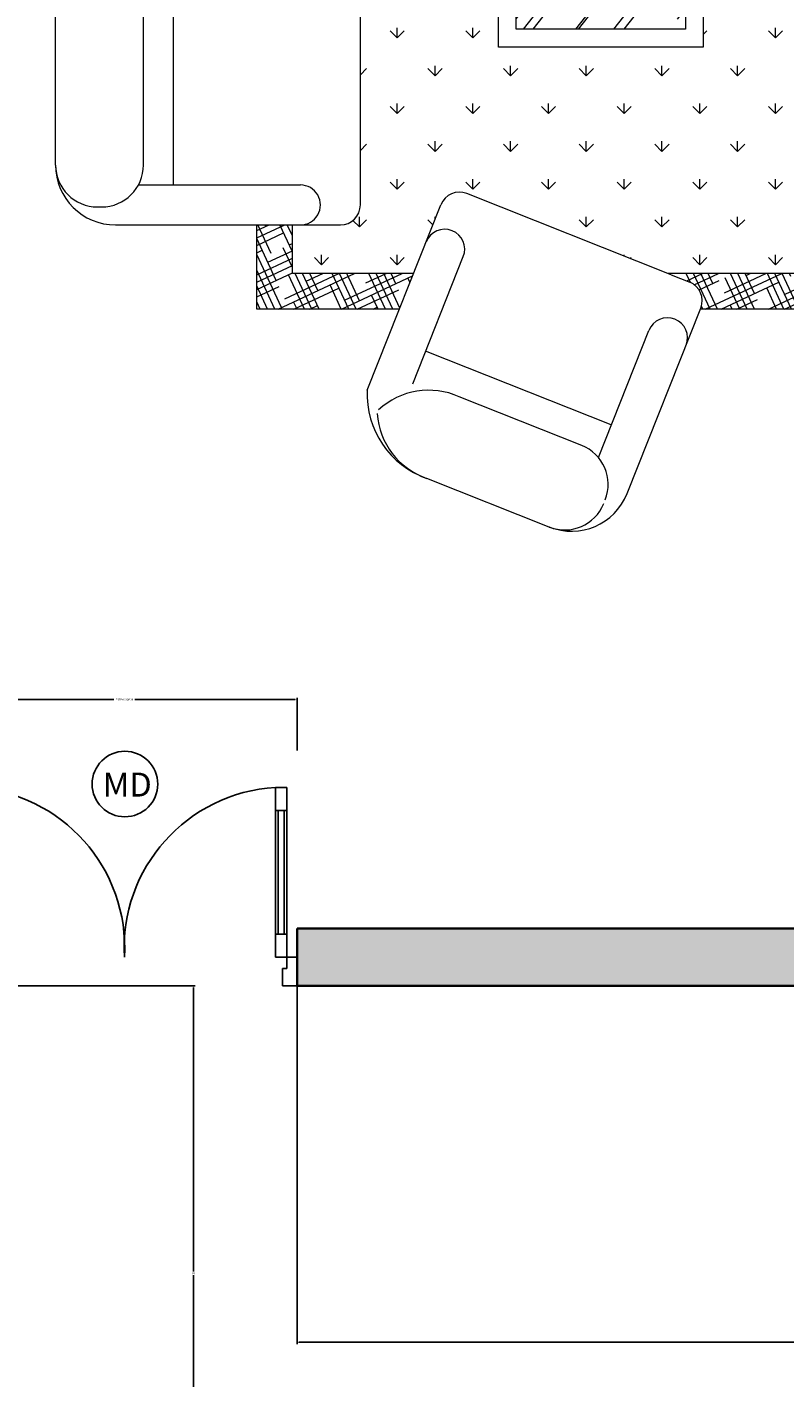
# Model space of a CAD drawing. Units: inches. Extents: x 2701 to 6846, y 811 to 2447.
# Tile 4 of 20: x 2944 to 3023, y 989 to 1130. Entities that reach past the tile are written whole.
import ezdxf

# ---------------------------------------------------------------- set-up
doc = ezdxf.new("R2010")
doc.units = ezdxf.units.IN
for name, color, linetype, lineweight in [('A-ANNO-DIMS', 2, 'Continuous', 18), ('A-DOOR', 4, 'Continuous', 25), ('A-FURN', 8, 'Continuous', 13), ('A-WALL', 7, 'Continuous', 35)]:
    doc.layers.add(name, color=color, linetype=linetype, lineweight=lineweight)
doc.layers.add('A-WALL-PATT', color=18, linetype='Continuous', lineweight=13, true_color=0x000000)
doc.styles.get("Standard").update_dxf_attribs({"font": 'arial.ttf'})
doc.dimstyles.get("Standard").update_dxf_attribs({"dimtxt": 0.18, "dimasz": 0.18, "dimexe": 0.18, "dimexo": 0.0625, "dimgap": 0.09, "dimtad": 0, "dimtih": 1, "dimtoh": 1, "dimdec": 4, "dimzin": 0, "dimdsep": 46, "dimtxsty": 'Standard', "dimcen": 0.09, "dimadec": 0, "dimazin": 0, "dimtfac": 1, "dimtdec": 4, "dimtofl": 0, "dimtmove": 0, "dimatfit": 3, "dimfxl": 1, "dimtolj": 1, "dimtzin": 0, "dimarcsym": 0})

# ---------------------------------------------------------------- blocks, each defined once
blk = doc.blocks.new('A$C09A905BE')
for p, q in [((35, 690), (35, 610)), ((75, 690), (35, 690)), ((75, 610), (75, 690)), ((1125, 690), (1125, 610)), ((1165, 690), (1125, 690)), ((1165, 610), (1165, 690)), ((35, 610), (75, 610)), ((35, 180), (35, 610)), ((35, 610), (75, 610)), ((45, 180), (45, 610)), ((45, 610), (65, 610)), ((65, 610), (65, 180)), ((75, 610), (75, 180)), ((1125, 610), (1165, 610)), ((1125, 180), (1125, 610)), ((1125, 610), (1165, 610)), ((1135, 180), (1135, 610)), ((1135, 610), (1155, 610)), ((1155, 610), (1155, 180)), ((1165, 610), (1165, 180)), ((35, 100), (35, 180)), ((35, 180), (75, 180)), ((75, 180), (35, 180)), ((65, 180), (45, 180)), ((75, 180), (75, 100)), ((1125, 100), (1125, 180)), ((1125, 180), (1165, 180)), ((1165, 180), (1125, 180)), ((1155, 180), (1135, 180)), ((1165, 180), (1165, 100)), ((0, 0), (0, 100)), ((0, 100), (35, 100)), ((35, 100), (35, 60)), ((75, 100), (35, 100)), ((1165, 100), (1125, 100)), ((1165, 100), (1200, 100)), ((1165, 60), (1165, 100)), ((1200, 100), (1200, 0)), ((35, 60), (50, 60)), ((50, 60), (50, 50)), ((50, 50), (50, 0)), ((1150, 50), (1150, 60)), ((1150, 60), (1165, 60)), ((1150, 0), (1150, 50)), ((50, 0), (0, 0)), ((1200, 0), (1150, 0))]:
    blk.add_line(p, q)
for centre, start, end in [((42.5, 132.5), 356.6637, 86.6637), ((1157.5, 132.5), 93.3363, 183.3363)]:
    blk.add_arc(centre, 558.4, start, end)
blk = doc.blocks.new('MAIN DOOR')
blk.add_circle((3420.7, 1223.43), 3.42)
at = {"xscale": 0.03, "yscale": 0.03, "zscale": 0.03}
blk.add_blockref('A$C09A905BE', (3402.65, 1202.37), dxfattribs=at)
at = {"insert": (3418.39, 1224.62), "char_height": 2.5, "attachment_point": 1}
blk.add_mtext('MD', dxfattribs=at)
blk = doc.blocks.new('A$C0782773B')
for p, q in [((1027.2, 2344.2), (2528, 2344.2)), ((1508.8, 2344.2), (1508.8, 1489.7)), ((2046.4, 2344.2), (2046.4, 1489.7)), ((3223.5, 2286.1), (2888.9, 2183.3)), ((3429.1, 1617), (3223.5, 2286.1)), ((3197, 2236.1), (2938.9, 2156.8)), ((3379.1, 1643.5), (3197, 2236.1)), ((909.6, 2226.6), (909.6, 2215.4)), ((2645.6, 2226.6), (2645.6, 2215.4)), ((859.2, 2176.2), (859.2, 1545.7)), ((2696, 2176.2), (2696, 1545.7)), ((2888.9, 2183.3), (3094.6, 1514.2)), ((2938.9, 2156.8), (3121.1, 1564.2)), ((971.2, 2111.9), (971.2, 1657.7)), ((1027.2, 2097.8), (2528, 2097.8)), ((2584, 2111.9), (2584, 1657.7)), ((971.2, 2013.8), (2584, 2013.8)), ((622.9, 1770.7), (643.4, 1780.2)), ((622.9, 1750), (687.8, 1780.2)), ((622.9, 1729.3), (732.1, 1780.2)), ((622.9, 1380.2), (622.9, 1780.2)), ((622.9, 1780.2), (859.2, 1780.2)), ((627.3, 1710.7), (776.5, 1780.2)), ((636.3, 1780.2), (637.5, 1777.5)), ((657, 1780.2), (686.2, 1717.5)), ((677.6, 1780.2), (724.3, 1680.2)), ((698.3, 1780.2), (745, 1680.2)), ((703.2, 1725.4), (820.8, 1780.2)), ((719, 1780.2), (765.7, 1680.2)), ((754.2, 1749.2), (786.3, 1680.2)), ((779.1, 1740.1), (859.2, 1777.4)), ((781.1, 1780.2), (788.2, 1765)), ((801.8, 1780.2), (836.9, 1705)), ((822.5, 1780.2), (859.2, 1701.5)), ((843.2, 1780.2), (859.2, 1745.8)), ((855, 1754.8), (859.2, 1756.8)), ((2696, 1682.3), (2906.1, 1780.2)), ((2696, 1780.2), (3012.8, 1780.2)), ((2696, 1703), (2835, 1767.8)), ((2696, 1755.4), (2731, 1680.2)), ((2696, 1723.7), (2759.1, 1753.1)), ((2717.2, 1754.3), (2751.7, 1680.2)), ((2736, 1680.2), (2950.4, 1780.2)), ((2746.5, 1780.2), (2751.2, 1770.1)), ((2767.2, 1780.2), (2799.9, 1710.1)), ((2787.9, 1780.2), (2834.5, 1680.2)), ((2790.8, 1685.1), (2994.8, 1780.2)), ((2808.5, 1780.2), (2855.2, 1680.2)), ((2829.2, 1780.2), (2875.9, 1680.2)), ((2866.7, 1699.8), (3016.1, 1769.5)), ((2891.3, 1780.2), (2901.9, 1757.6)), ((2912, 1780.2), (2950.5, 1697.6)), ((2932.7, 1780.2), (2999.2, 1637.5)), ((2942.6, 1714.5), (3021.7, 1751.4)), ((2953.4, 1780.2), (3039.7, 1595.1)), ((2974, 1780.2), (3039.7, 1639.5)), ((622.9, 1720.3), (722.9, 1505.8)), ((739.5, 1680.2), (795, 1706.1)), ((783.9, 1680.2), (859.2, 1715.4)), ((2696, 1711), (2710.4, 1680.2)), ((2867.9, 1741.8), (2896.6, 1680.2)), ((3018.5, 1729.2), (3027.2, 1733.3)), ((3018.5, 1729.2), (3039.7, 1683.9)), ((622.9, 1646.6), (719.1, 1691.4)), ((622.9, 1667.2), (643.2, 1676.7)), ((622.9, 1675.9), (681.6, 1549.8)), ((622.9, 1625.9), (722.9, 1672.5)), ((652.2, 1701.6), (722.9, 1550.2)), ((722.9, 1340.4), (722.9, 1680.2)), ((722.9, 1680.2), (859.2, 1680.2)), ((802.9, 1689.1), (807, 1680.2)), ((828.2, 1680.2), (859.2, 1694.7)), ((2696, 1680.2), (2939.7, 1680.2)), ((2765.9, 1694.2), (2772.4, 1680.2)), ((2916.6, 1681.7), (2917.2, 1680.2)), ((2939.7, 1651.1), (3034.4, 1695.3)), ((2939.7, 1671.8), (2958.5, 1680.6)), ((2939.7, 1680.2), (2939.7, 1461.7)), ((2939.7, 1630.4), (3039.7, 1677.1)), ((3039.7, 1692.8), (3039.7, 1461.7)), ((622.9, 1605.2), (722.9, 1651.8)), ((622.9, 1631.5), (633, 1609.9)), ((674.9, 1608.7), (722.9, 1631.1)), ((700.9, 1641.6), (722.9, 1594.5)), ((2939.7, 1609.7), (3039.7, 1656.4)), ((2939.7, 1632.1), (3019.1, 1461.7)), ((2990.2, 1612.6), (3039.7, 1635.7)), ((3121.1, 1564.2), (3379.1, 1643.5)), ((747.4, 1598.5), (767.3, 1618.4)), ((747.4, 1598.5), (775.6, 1598.5)), ((747.4, 1598.5), (767.3, 1578.6)), ((2868.8, 1598.5), (2888.7, 1618.4)), ((2868.8, 1598.5), (2896.9, 1598.5)), ((2868.8, 1598.5), (2888.7, 1578.6)), ((2965.3, 1621.7), (3039.7, 1462)), ((3094.6, 1514.2), (3429.1, 1617)), ((622.9, 1543.1), (690.7, 1574.7)), ((622.9, 1522.4), (722.9, 1569.1)), ((2939.7, 1587.7), (2994.7, 1469.9)), ((2939.7, 1547.7), (3006, 1578.6)), ((2939.7, 1527), (3039.7, 1573.6)), ((3013.9, 1561.6), (3039.7, 1506.4)), ((622.9, 1501.7), (722.9, 1548.4)), ((622.9, 1542.8), (715.9, 1343.2)), ((646.5, 1492.1), (722.9, 1527.7)), ((647.7, 1534), (722.9, 1372.7)), ((2939.7, 1506.3), (3039.7, 1552.9)), ((2939.7, 1543.4), (2946, 1529.9)), ((2961.8, 1495.9), (3039.7, 1532.2)), ((622.9, 1498.4), (677.1, 1382.2)), ((722.4, 1506.8), (722.9, 1507)), ((853.5, 1492.5), (871.6, 1510.6)), ((853.5, 1492.5), (881.6, 1492.5)), ((853.5, 1492.5), (873.4, 1472.6)), ((915.2, 1489.7), (2640, 1489.7)), ((1068.4, 1489.7), (1085.5, 1472.6)), ((1280.5, 1489.7), (1297.7, 1472.6)), ((1492.7, 1489.7), (1509.8, 1472.6)), ((1704.8, 1489.7), (1721.9, 1472.6)), ((1916.9, 1489.7), (1934.1, 1472.6)), ((2129.1, 1489.7), (2146.2, 1472.6)), ((2341.2, 1489.7), (2358.3, 1472.6)), ((2553.3, 1489.7), (2570.5, 1472.6)), ((2762.7, 1492.5), (2782.6, 1512.3)), ((2762.7, 1492.5), (2790.8, 1492.5)), ((2762.7, 1492.5), (2782.6, 1472.6)), ((3037.7, 1510.6), (3039.7, 1511.5)), ((395.3, 1470.7), (915.7, 1263.8)), ((622.9, 1419), (722.9, 1465.6)), ((622.9, 1439.7), (662.4, 1458.1)), ((622.9, 1454.1), (628.4, 1442.2)), ((622.9, 1398.3), (722.9, 1444.9)), ((696.4, 1473.9), (722.9, 1417.1)), ((3326.7, 1461.7), (2766.7, 1461.7)), ((2977.2, 1461.7), (2977.7, 1461.9)), ((3021.6, 1461.7), (3039.7, 1470.2)), ((625.9, 1379), (722.9, 1424.2)), ((694.1, 1390.1), (722.9, 1403.5)), ((747.4, 1386.4), (767.3, 1406.3)), ((959.6, 1386.4), (979.5, 1406.3)), ((1171.7, 1386.4), (1191.6, 1406.3)), ((1383.8, 1386.4), (1403.7, 1406.3)), ((1596, 1386.4), (1615.9, 1406.3)), ((1808.1, 1386.4), (1828, 1406.3)), ((2020.2, 1386.4), (2040.1, 1406.3)), ((2232.4, 1386.4), (2252.3, 1406.3)), ((2444.5, 1386.4), (2464.4, 1406.3)), ((2656.6, 1386.4), (2676.5, 1406.3)), ((2710.7, 1349.7), (2710.7, 1405.7)), ((747.4, 1386.4), (775.6, 1386.4)), ((747.4, 1386.4), (767.3, 1366.5)), ((959.6, 1386.4), (987.7, 1386.4)), ((959.6, 1386.4), (979.5, 1366.5)), ((1171.7, 1386.4), (1199.8, 1386.4)), ((1171.7, 1386.4), (1191.6, 1366.5)), ((1383.8, 1386.4), (1412, 1386.4)), ((1383.8, 1386.4), (1403.7, 1366.5)), ((1596, 1386.4), (1624.1, 1386.4)), ((1596, 1386.4), (1615.9, 1366.5)), ((1808.1, 1386.4), (1836.2, 1386.4)), ((1808.1, 1386.4), (1828, 1366.5)), ((2020.2, 1386.4), (2048.4, 1386.4)), ((2020.2, 1386.4), (2040.1, 1366.5)), ((2232.4, 1386.4), (2260.5, 1386.4)), ((2232.4, 1386.4), (2252.3, 1366.5)), ((2444.5, 1386.4), (2472.6, 1386.4)), ((2444.5, 1386.4), (2464.4, 1366.5)), ((2656.6, 1386.4), (2684.8, 1386.4)), ((2656.6, 1386.4), (2676.5, 1366.5)), ((413.6, 1342.9), (770.2, 1201.1)), ((697.7, 1350.4), (709.9, 1356.1)), ((721.7, 1340.9), (722.9, 1341.5)), ((2710.7, 1349.7), (2710.7, 733.3)), ((3262.5, 1349.7), (2878.7, 1349.7)), ((3164.3, 1349.7), (3164.3, 789.3)), ((11.5, 960), (148, 1303.4)), ((297.8, 785.9), (504.9, 1306.6)), ((859.4, 1286.2), (873.4, 1300.2)), ((1065.6, 1280.3), (1085.5, 1300.2)), ((1277.8, 1280.3), (1297.7, 1300.2)), ((1489.9, 1280.3), (1509.8, 1300.2)), ((1702, 1280.3), (1721.9, 1300.2)), ((1914.2, 1280.3), (1934.1, 1300.2)), ((2126.3, 1280.3), (2146.2, 1300.2)), ((2338.4, 1280.3), (2358.3, 1300.2)), ((2550.6, 1280.3), (2570.5, 1300.2)), ((3248.3, 1293.7), (3248.3, 924.1)), ((3494.7, 1293.7), (3494.7, 924.1)), ((874.1, 1280.3), (881.6, 1280.3)), ((1065.6, 1280.3), (1093.8, 1280.3)), ((1065.6, 1280.3), (1085.5, 1260.4)), ((1277.8, 1280.3), (1305.9, 1280.3)), ((1277.8, 1280.3), (1297.7, 1260.4)), ((1489.9, 1280.3), (1518, 1280.3)), ((1489.9, 1280.3), (1509.8, 1260.4)), ((1702, 1280.3), (1730.2, 1280.3)), ((1702, 1280.3), (1721.9, 1260.4)), ((1914.2, 1280.3), (1942.3, 1280.3)), ((1914.2, 1280.3), (1934.1, 1260.4)), ((2126.3, 1280.3), (2154.4, 1280.3)), ((2126.3, 1280.3), (2146.2, 1260.4)), ((2338.4, 1280.3), (2366.6, 1280.3)), ((2338.4, 1280.3), (2358.3, 1260.4)), ((2550.6, 1280.3), (2578.7, 1280.3)), ((2550.6, 1280.3), (2570.5, 1260.4)), ((240.4, 868.9), (377, 1212.4)), ((719.3, 618.3), (947, 1191)), ((959.6, 1174.3), (979.5, 1194.1)), ((1171.7, 1174.3), (1191.6, 1194.1)), ((1383.8, 1174.3), (1403.7, 1194.1)), ((1596, 1174.3), (1615.9, 1194.1)), ((1808.1, 1174.3), (1828, 1194.1)), ((2020.2, 1174.3), (2040.1, 1194.1)), ((2232.4, 1174.3), (2252.3, 1194.1)), ((2444.5, 1174.3), (2464.4, 1194.1)), ((2656.6, 1174.3), (2676.5, 1194.1)), ((959.6, 1174.3), (987.7, 1174.3)), ((959.6, 1174.3), (979.5, 1154.4)), ((1171.7, 1174.3), (1199.8, 1174.3)), ((1171.7, 1174.3), (1191.6, 1154.4)), ((1383.8, 1174.3), (1412, 1174.3)), ((1383.8, 1174.3), (1403.7, 1154.4)), ((1596, 1174.3), (1624.1, 1174.3)), ((1596, 1174.3), (1615.9, 1154.4)), ((1808.1, 1174.3), (1836.2, 1174.3)), ((1808.1, 1174.3), (1828, 1154.4)), ((2020.2, 1174.3), (2048.4, 1174.3)), ((2020.2, 1174.3), (2040.1, 1154.4)), ((2232.4, 1174.3), (2260.5, 1174.3)), ((2232.4, 1174.3), (2252.3, 1154.4)), ((2444.5, 1174.3), (2472.6, 1174.3)), ((2444.5, 1174.3), (2464.4, 1154.4)), ((2656.6, 1174.3), (2684.8, 1174.3)), ((2656.6, 1174.3), (2676.5, 1154.4)), ((1358.2, 528.2), (1358.2, 1102.6)), ((1358.2, 1102.6), (2266.7, 1102.6)), ((2266.7, 1102.6), (2266.7, 528.2)), ((1065.6, 1068.2), (1085.5, 1088.1)), ((1065.6, 1068.2), (1093.8, 1068.2)), ((1065.6, 1068.2), (1085.5, 1048.3)), ((1277.8, 1068.2), (1297.7, 1088.1)), ((1277.8, 1068.2), (1305.9, 1068.2)), ((1277.8, 1068.2), (1297.7, 1048.3)), ((2338.4, 1068.2), (2358.3, 1088.1)), ((2338.4, 1068.2), (2366.6, 1068.2)), ((2338.4, 1068.2), (2358.3, 1048.3)), ((2550.6, 1068.2), (2570.5, 1088.1)), ((2550.6, 1068.2), (2578.7, 1068.2)), ((2550.6, 1068.2), (2570.5, 1048.3)), ((1408.2, 578.2), (1408.2, 1052.6)), ((1408.2, 1052.6), (2216.7, 1052.6)), ((1408.2, 1031.9), (1644.7, 847.1)), ((1437.7, 1052.6), (1999.3, 613.9)), ((1510.8, 1052.6), (2118.1, 578.2)), ((1674, 1052.6), (1887.9, 885.5)), ((1681.3, 1052.6), (2216.7, 634.3)), ((1738, 1027.4), (2092.6, 750.4)), ((1837.3, 1052.6), (1926.1, 983.2)), ((1925, 1052.6), (2216.7, 824.7)), ((2000.5, 1052.6), (2216.7, 883.7)), ((2029.7, 1052.6), (2097.2, 999.9)), ((2163.7, 1052.6), (2215.4, 1012.3)), ((2168.6, 1052.6), (2216.7, 1015)), ((2216.7, 1052.6), (2216.7, 578.2)), ((1408.2, 1005.3), (1598.7, 856.4)), ((959.6, 962.1), (979.5, 982)), ((959.6, 962.1), (987.7, 962.1)), ((959.6, 962.1), (979.5, 942.2)), ((1171.7, 962.1), (1191.6, 982)), ((1171.7, 962.1), (1199.8, 962.1)), ((1171.7, 962.1), (1191.6, 942.2)), ((2136.2, 969.5), (2216.7, 906.5)), ((2444.5, 962.1), (2464.4, 982)), ((2444.5, 962.1), (2472.6, 962.1)), ((2444.5, 962.1), (2464.4, 942.2)), ((2656.6, 962.1), (2676.5, 982)), ((2656.6, 962.1), (2684.8, 962.1)), ((2656.6, 962.1), (2676.5, 942.2)), ((853.5, 856.1), (873.4, 876)), ((1065.6, 856.1), (1085.5, 876)), ((1277.8, 856.1), (1297.7, 876)), ((1408.2, 885.3), (1646.9, 698.8)), ((1408.2, 877.7), (1560.4, 758.8)), ((2338.4, 856.1), (2358.3, 876)), ((2550.6, 856.1), (2570.5, 876)), ((853.5, 856.1), (881.6, 856.1)), ((853.5, 856.1), (873.4, 836.2)), ((1065.6, 856.1), (1093.8, 856.1)), ((1065.6, 856.1), (1085.5, 836.2)), ((1277.8, 856.1), (1305.9, 856.1)), ((1277.8, 856.1), (1297.7, 836.2)), ((2091.6, 853.9), (2216.7, 756.2)), ((2338.4, 856.1), (2366.6, 856.1)), ((2338.4, 856.1), (2358.3, 836.2)), ((2550.6, 856.1), (2578.7, 856.1)), ((2550.6, 856.1), (2570.5, 836.2)), ((206.6, 822.1), (563.2, 680.3)), ((959.6, 750), (979.5, 769.9)), ((1171.7, 750), (1191.6, 769.9)), ((1408.2, 778.7), (1640.1, 597.6)), ((1733.4, 777.9), (1989, 578.2)), ((2006.1, 793.2), (2216.7, 628.6)), ((2444.5, 750), (2464.4, 769.9)), ((2656.6, 750), (2676.5, 769.9)), ((3262.5, 789.3), (2878.7, 789.3)), ((105.5, 741.8), (625.9, 534.9)), ((764.8, 732.7), (767.3, 730.1)), ((771.7, 750), (775.6, 750)), ((959.6, 750), (987.7, 750)), ((959.6, 750), (979.5, 730.1)), ((1171.7, 750), (1199.8, 750)), ((1171.7, 750), (1191.6, 730.1)), ((1408.2, 750.2), (1628.4, 578.2)), ((1764.2, 727.1), (1954.8, 578.2)), ((2131.6, 719.9), (2216.7, 653.4)), ((2444.5, 750), (2472.6, 750)), ((2444.5, 750), (2464.4, 730.1)), ((2656.6, 750), (2684.8, 750)), ((2656.6, 750), (2676.5, 730.1)), ((853.5, 643.9), (873.4, 663.8)), ((1065.6, 643.9), (1085.5, 663.8)), ((1277.8, 643.9), (1297.7, 663.8)), ((1678.6, 666.4), (1791.6, 578.2)), ((2338.4, 643.9), (2358.3, 663.8)), ((2550.6, 643.9), (2570.5, 663.8)), ((2762.7, 643.9), (2782.6, 663.8)), ((3326.7, 677.3), (2766.7, 677.3)), ((2939.7, 658.1), (2981, 677.3)), ((2939.7, 637.4), (3025.4, 677.3)), ((2939.7, 677.3), (2939.7, 567.7)), ((2939.7, 616.7), (3039.7, 663.3)), ((2950.4, 677.3), (2971.8, 631.6)), ((2971.1, 677.3), (3020.4, 571.6)), ((2991.8, 677.3), (3039.7, 574.7)), ((3012.5, 677.3), (3039.7, 619.1)), ((3039.7, 677.3), (3039.7, 567.7)), ((719.3, 618.3), (698.6, 566.2)), ((722.9, 100), (722.9, 627.2)), ((853.5, 643.9), (881.6, 643.9)), ((853.5, 643.9), (873.4, 624)), ((1065.6, 643.9), (1093.8, 643.9)), ((1065.6, 643.9), (1085.5, 624)), ((1277.8, 643.9), (1305.9, 643.9)), ((1277.8, 643.9), (1297.7, 624)), ((2338.4, 643.9), (2366.6, 643.9)), ((2338.4, 643.9), (2358.3, 624)), ((2550.6, 643.9), (2578.7, 643.9)), ((2550.6, 643.9), (2570.5, 624)), ((2762.7, 643.9), (2790.8, 643.9)), ((2762.7, 643.9), (2782.6, 624)), ((2939.7, 611.7), (2960.2, 567.7)), ((2962.7, 606.7), (3039.7, 642.6)), ((3038.6, 621.4), (3039.7, 621.9)), ((697.8, 564.3), (722.9, 576)), ((701.9, 574.6), (722.9, 529.8)), ((722.1, 575.7), (722.9, 574.1)), ((2216.7, 578.2), (1408.2, 578.2)), ((1436.7, 600.4), (1465.1, 578.2)), ((1530.9, 599.1), (1557.7, 578.2)), ((2967.7, 567.7), (2978.5, 572.7)), ((3012, 567.7), (3039.7, 580.6)), ((622.9, 508.7), (722.9, 555.3)), ((622.9, 0), (622.9, 536.1)), ((622.9, 488), (722.9, 534.6)), ((622.9, 529.4), (630.9, 533.1)), ((676.8, 539.8), (702.9, 483.9)), ((691.3, 553.2), (722.9, 485.4)), ((747.4, 537.9), (767.3, 557.8)), ((747.4, 537.9), (775.6, 537.9)), ((747.4, 537.9), (767.3, 518)), ((959.6, 537.9), (979.5, 557.8)), ((959.6, 537.9), (987.7, 537.9)), ((959.6, 537.9), (979.5, 518)), ((1171.7, 537.9), (1191.6, 557.8)), ((1171.7, 537.9), (1199.8, 537.9)), ((1171.7, 537.9), (1191.6, 518)), ((2444.5, 537.9), (2464.4, 557.8)), ((2444.5, 537.9), (2472.6, 537.9)), ((2444.5, 537.9), (2464.4, 518)), ((2656.6, 537.9), (2676.5, 557.8)), ((2656.6, 537.9), (2684.8, 537.9)), ((2656.6, 537.9), (2676.5, 518)), ((2868.8, 537.9), (2873.3, 542.4)), ((2868.8, 537.9), (2873.3, 537.9)), ((2868.8, 537.9), (2873.3, 533.3)), ((2873.3, 567.7), (3323.3, 567.7)), ((2873.3, 117.7), (2873.3, 567.7)), ((3323.3, 567.7), (3323.3, 117.7)), ((622.9, 522.4), (722.9, 307.9)), ((694.9, 500.9), (722.9, 513.9)), ((2266.7, 528.2), (1358.2, 528.2)), ((1393.5, 528.2), (1403.7, 518)), ((1605.7, 528.2), (1615.9, 518)), ((1817.8, 528.2), (1828, 518)), ((2029.9, 528.2), (2040.1, 518)), ((2242.1, 528.2), (2252.3, 518)), ((3098.3, 156.5), (3098.3, 526.4)), ((622.9, 478), (698.3, 316.3)), ((622.9, 425.9), (710.8, 466.9)), ((668.9, 468.1), (722.9, 352.3)), ((622.9, 446.6), (634.9, 452.2)), ((622.9, 405.3), (722.9, 451.9)), ((622.9, 433.6), (649.6, 376.3)), ((622.9, 384.6), (722.9, 431.2)), ((853.5, 431.8), (873.4, 451.7)), ((853.5, 431.8), (881.6, 431.8)), ((853.5, 431.8), (873.4, 411.9)), ((1065.6, 431.8), (1085.5, 451.7)), ((1065.6, 431.8), (1093.8, 431.8)), ((1065.6, 431.8), (1085.5, 411.9)), ((1277.8, 431.8), (1297.7, 451.7)), ((1277.8, 431.8), (1305.9, 431.8)), ((1277.8, 431.8), (1297.7, 411.9)), ((1489.9, 431.8), (1509.8, 451.7)), ((1489.9, 431.8), (1518, 431.8)), ((1489.9, 431.8), (1509.8, 411.9)), ((1702, 431.8), (1721.9, 451.7)), ((1702, 431.8), (1730.2, 431.8)), ((1702, 431.8), (1721.9, 411.9)), ((1914.2, 431.8), (1934.1, 451.7)), ((1914.2, 431.8), (1942.3, 431.8)), ((1914.2, 431.8), (1934.1, 411.9)), ((2126.3, 431.8), (2146.2, 451.7)), ((2126.3, 431.8), (2154.4, 431.8)), ((2126.3, 431.8), (2146.2, 411.9)), ((2338.4, 431.8), (2358.3, 451.7)), ((2338.4, 431.8), (2366.6, 431.8)), ((2338.4, 431.8), (2358.3, 411.9)), ((2550.6, 431.8), (2570.5, 451.7)), ((2550.6, 431.8), (2578.7, 431.8)), ((2550.6, 431.8), (2570.5, 411.9)), ((2762.7, 431.8), (2782.6, 451.7)), ((2762.7, 431.8), (2790.8, 431.8)), ((2762.7, 431.8), (2782.6, 411.9)), ((666.6, 384.3), (722.9, 410.5)), ((717.6, 408), (722.9, 396.7)), ((622.9, 322.5), (682.4, 350.3)), ((622.9, 301.8), (722.9, 348.4)), ((622.9, 344.9), (722.9, 130.5)), ((747.4, 325.7), (767.3, 345.6)), ((959.6, 325.7), (979.5, 345.6)), ((1171.7, 325.7), (1191.6, 345.6)), ((1383.8, 325.7), (1403.7, 345.6)), ((1596, 325.7), (1615.9, 345.6)), ((1808.1, 325.7), (1828, 345.6)), ((2020.2, 325.7), (2040.1, 345.6)), ((2232.4, 325.7), (2252.3, 345.6)), ((2444.5, 325.7), (2464.4, 345.6)), ((2656.6, 325.7), (2676.5, 345.6)), ((2914.5, 342.7), (3284.1, 342.7)), ((622.9, 281.1), (722.9, 327.8)), ((638.2, 267.6), (722.9, 307.1)), ((747.4, 325.7), (775.6, 325.7)), ((747.4, 325.7), (767.3, 305.8)), ((959.6, 325.7), (987.7, 325.7)), ((959.6, 325.7), (979.5, 305.8)), ((1171.7, 325.7), (1199.8, 325.7)), ((1171.7, 325.7), (1191.6, 305.8)), ((1383.8, 325.7), (1412, 325.7)), ((1383.8, 325.7), (1403.7, 305.8)), ((1596, 325.7), (1624.1, 325.7)), ((1596, 325.7), (1615.9, 305.8)), ((1808.1, 325.7), (1836.2, 325.7)), ((1808.1, 325.7), (1828, 305.8)), ((2020.2, 325.7), (2048.4, 325.7)), ((2020.2, 325.7), (2040.1, 305.8)), ((2232.4, 325.7), (2260.5, 325.7)), ((2232.4, 325.7), (2252.3, 305.8)), ((2444.5, 325.7), (2472.6, 325.7)), ((2444.5, 325.7), (2464.4, 305.8)), ((2656.6, 325.7), (2684.8, 325.7)), ((2656.6, 325.7), (2676.5, 305.8)), ((2868.8, 325.7), (2873.3, 330.3)), ((2868.8, 325.7), (2873.3, 325.7)), ((2868.8, 325.7), (2873.3, 321.2)), ((622.9, 300.5), (693.7, 148.6)), ((664.3, 300.4), (722.9, 174.8)), ((714.1, 282.3), (722.9, 286.4)), ((622.9, 256.2), (645, 208.7)), ((622.9, 198.4), (722.9, 245)), ((622.9, 219.1), (654.1, 233.6)), ((713, 240.4), (722.9, 219.2)), ((853.5, 219.7), (873.4, 239.6)), ((1065.6, 219.7), (1085.5, 239.6)), ((1277.8, 219.7), (1297.7, 239.6)), ((1489.9, 219.7), (1509.8, 239.6)), ((1702, 219.7), (1721.9, 239.6)), ((1914.2, 219.7), (1934.1, 239.6)), ((2126.3, 219.7), (2146.2, 239.6)), ((2338.4, 219.7), (2358.3, 239.6)), ((2550.6, 219.7), (2570.5, 239.6)), ((2762.7, 219.7), (2782.6, 239.6)), ((622.9, 177.7), (722.9, 224.3)), ((622.9, 157), (722.9, 203.6)), ((853.5, 219.7), (881.6, 219.7)), ((853.5, 219.7), (873.4, 199.8)), ((1065.6, 219.7), (1093.8, 219.7)), ((1065.6, 219.7), (1085.5, 199.8)), ((1277.8, 219.7), (1305.9, 219.7)), ((1277.8, 219.7), (1297.7, 199.8)), ((1489.9, 219.7), (1518, 219.7)), ((1489.9, 219.7), (1509.8, 199.8)), ((1702, 219.7), (1730.2, 219.7)), ((1702, 219.7), (1721.9, 199.8)), ((1914.2, 219.7), (1942.3, 219.7)), ((1914.2, 219.7), (1934.1, 199.8)), ((2126.3, 219.7), (2154.4, 219.7)), ((2126.3, 219.7), (2146.2, 199.8)), ((2338.4, 219.7), (2366.6, 219.7)), ((2338.4, 219.7), (2358.3, 199.8)), ((2550.6, 219.7), (2578.7, 219.7)), ((2550.6, 219.7), (2570.5, 199.8)), ((2762.7, 219.7), (2790.8, 219.7)), ((2762.7, 219.7), (2782.6, 199.8)), ((622.9, 167.4), (700.9, 0)), ((685.8, 165.6), (722.9, 182.9)), ((622.9, 94.9), (701.6, 131.7)), ((622.9, 123.1), (680.3, 0)), ((622.9, 74.2), (722.9, 120.9)), ((622.9, 115.6), (625.7, 116.9)), ((659.7, 132.8), (721.6, 0)), ((747.4, 113.6), (767.3, 133.5)), ((959.6, 113.6), (979.5, 133.5)), ((1171.7, 113.6), (1191.6, 133.5)), ((1383.8, 113.6), (1403.7, 133.5)), ((1596, 113.6), (1615.9, 133.5)), ((1808.1, 113.6), (1828, 133.5)), ((2020.2, 113.6), (2040.1, 133.5)), ((2232.4, 113.6), (2252.3, 133.5)), ((2444.5, 113.6), (2464.4, 133.5)), ((2656.6, 113.6), (2676.5, 133.5)), ((2745, 8.7), (2978.7, 117.7)), ((2820.9, 23.4), (3023, 117.7)), ((2868.8, 113.6), (2873.3, 118.1)), ((3323.3, 117.7), (2873.3, 117.7)), ((2939.7, 117.7), (2939.7, 100)), ((2983.9, 117.7), (3006.7, 68.7)), ((3004.5, 117.7), (3039.7, 42.3)), ((3025.2, 117.7), (3039.7, 86.7)), ((3039.7, 117.7), (3039.7, 0)), ((622.9, 53.5), (722.9, 100.2)), ((622.9, 78.7), (640.4, 41)), ((657.4, 49), (766.8, 100)), ((2939.7, 100), (722.9, 100)), ((733.3, 63.7), (811.2, 100)), ((737.1, 100), (742.4, 88.6)), ((747.4, 113.6), (775.6, 113.6)), ((747.4, 113.6), (761, 100)), ((757.8, 100), (791.1, 28.5)), ((778.4, 100), (825.1, 0)), ((799.1, 100), (845.8, 0)), ((809.2, 78.4), (855.6, 100)), ((819.8, 100), (866.5, 0)), ((863, 0), (1052.8, 88.5)), ((881.9, 100), (893, 76.1)), ((885.1, 93.1), (899.9, 100)), ((902.6, 100), (941.7, 16)), ((907.3, 0), (1121.8, 100)), ((923.3, 100), (969.9, 0)), ((943.9, 100), (990.6, 0)), ((951.7, 0), (1166.1, 100)), ((959.6, 113.6), (987.7, 113.6)), ((959.6, 113.6), (973.2, 100)), ((964.6, 100), (1011.3, 0)), ((1008.6, 5.8), (1210.5, 100)), ((1026.7, 100), (1043.7, 63.6)), ((1047.4, 100), (1092.4, 3.5)), ((1068.1, 100), (1114.7, 0)), ((1084.4, 20.5), (1254.9, 100)), ((1088.8, 100), (1135.4, 0)), ((1111.7, 95.3), (1156.1, 0)), ((1160.3, 35.2), (1299.2, 100)), ((1171.5, 100), (1194.3, 51.1)), ((1171.7, 113.6), (1199.8, 113.6)), ((1171.7, 113.6), (1185.3, 100)), ((1192.2, 100), (1238.8, 0)), ((1212.9, 100), (1259.5, 0)), ((1233.6, 100), (1280.2, 0)), ((1236.2, 49.9), (1343.6, 100)), ((1262.3, 82.8), (1300.9, 0)), ((1295.7, 100), (1296.3, 98.6)), ((1312.1, 64.6), (1388, 100)), ((1316.3, 100), (1345, 38.6)), ((1337, 100), (1383.7, 0)), ((1357.7, 100), (1404.3, 0)), ((1378.4, 100), (1425, 0)), ((1383.8, 113.6), (1412, 113.6)), ((1383.8, 113.6), (1397.4, 100)), ((1388, 79.3), (1432.3, 100)), ((1439.7, 0), (1631.6, 89.5)), ((1440.5, 100), (1446.9, 86.1)), ((1461.2, 100), (1495.6, 26.1)), ((1463.9, 94), (1476.7, 100)), ((1481.8, 100), (1528.5, 0)), ((1484.1, 0), (1698.5, 100)), ((1502.5, 100), (1549.2, 0)), ((1523.2, 100), (1569.9, 0)), ((1528.5, 0), (1742.9, 100)), ((1585.3, 100), (1597.6, 73.6)), ((1587.4, 6.8), (1787.3, 100)), ((1596, 113.6), (1624.1, 113.6)), ((1596, 113.6), (1609.6, 100)), ((1606, 100), (1646.3, 13.6)), ((1626.7, 100), (1673.3, 0)), ((1647.4, 100), (1694, 0)), ((1663.3, 21.5), (1831.6, 100)), ((1668, 100), (1714.7, 0)), ((1730.1, 100), (1748.2, 61.1)), ((1739.2, 36.2), (1876, 100)), ((1750.8, 100), (1796.9, 1.1)), ((1771.5, 100), (1818.1, 0)), ((1792.2, 100), (1838.8, 0)), ((1808.1, 113.6), (1836.2, 113.6)), ((1808.1, 113.6), (1821.7, 100)), ((1815.1, 50.9), (1920.4, 100)), ((1816.2, 92.8), (1859.5, 0)), ((1874.9, 100), (1898.9, 48.6)), ((1891, 65.6), (1964.7, 100)), ((1895.6, 100), (1942.2, 0)), ((1916.3, 100), (1962.9, 0)), ((1937, 100), (1983.6, 0)), ((1966.9, 80.3), (2009.1, 100)), ((1966.9, 80.3), (2004.3, 0)), ((1999.1, 100), (2000.8, 96.2)), ((2016.5, 0), (2210.4, 90.4)), ((2019.7, 100), (2049.5, 36.1)), ((2020.2, 113.6), (2048.4, 113.6)), ((2020.2, 113.6), (2033.8, 100)), ((2040.4, 100), (2087.1, 0)), ((2042.8, 95), (2053.5, 100)), ((2060.8, 0), (2275.3, 100)), ((2061.1, 100), (2107.8, 0)), ((2081.8, 100), (2128.4, 0)), ((2105.2, 0), (2319.7, 100)), ((2143.9, 100), (2151.5, 83.6)), ((2164.6, 100), (2200.2, 23.6)), ((2166.2, 7.8), (2364, 100)), ((2185.2, 100), (2231.9, 0)), ((2205.9, 100), (2252.6, 0)), ((2226.6, 100), (2273.3, 0)), ((2232.4, 113.6), (2260.5, 113.6)), ((2232.4, 113.6), (2246, 100)), ((2242.1, 22.5), (2408.4, 100)), ((2288.7, 100), (2302.1, 71.1)), ((2309.4, 100), (2350.8, 11.1)), ((2318, 37.2), (2452.8, 100)), ((2330.1, 100), (2376.7, 0)), ((2350.8, 100), (2397.4, 0)), ((2371.4, 100), (2418.1, 0)), ((2393.9, 51.9), (2497.1, 100)), ((2433.5, 100), (2452.8, 58.6)), ((2444.5, 113.6), (2472.6, 113.6)), ((2444.5, 113.6), (2458.1, 100)), ((2454.2, 100), (2500.8, 0)), ((2469.8, 66.6), (2541.5, 100)), ((2474.9, 100), (2521.5, 0)), ((2495.6, 100), (2542.2, 0)), ((2520.8, 90.3), (2562.9, 0)), ((2545.7, 81.3), (2585.9, 100)), ((2548.9, 0), (2713.3, 76.7)), ((2578.3, 100), (2603.4, 46.1)), ((2593.2, 0), (2789.2, 91.4)), ((2599, 100), (2645.6, 0)), ((2619.7, 100), (2666.3, 0)), ((2621.6, 96), (2630.2, 100)), ((2637.6, 0), (2852.1, 100)), ((2640.4, 100), (2687, 0)), ((2656.6, 113.6), (2684.8, 113.6)), ((2656.6, 113.6), (2670.2, 100)), ((2671.4, 77.8), (2707.7, 0)), ((2682, 0), (2896.4, 100)), ((2702.5, 100), (2705.4, 93.7)), ((2723.1, 100), (2754.1, 33.6)), ((2743.8, 100), (2790.5, 0)), ((2764.5, 100), (2811.2, 0)), ((2785.2, 100), (2831.8, 0)), ((2847.3, 100), (2856.1, 81.2)), ((2868, 100), (2904.7, 21.1)), ((2868.8, 113.6), (2896.9, 113.6)), ((2868.8, 113.6), (2882.4, 100)), ((2888.7, 100), (2935.3, 0)), ((2896.8, 38.1), (3039.7, 104.7)), ((2909.3, 100), (2956, 0)), ((2930, 100), (2976.7, 0)), ((2972.7, 52.8), (3039.7, 84.1)), ((708.4, 72.7), (742.3, 0)), ((729.9, 0), (825.1, 44.4)), ((774.2, 0), (901, 59.1)), ((818.6, 0), (976.9, 73.8)), ((859, 60.2), (887.1, 0)), ((1009.7, 47.7), (1032, 0)), ((1306.6, 0), (1403.9, 45.4)), ((1351, 0), (1479.8, 60.1)), ((1395.4, 0), (1555.7, 74.8)), ((1413, 70.3), (1445.7, 0)), ((1563.6, 57.8), (1590.5, 0)), ((1714.3, 45.3), (1735.4, 0)), ((1883.4, 0), (1982.7, 46.3)), ((1927.7, 0), (2058.6, 61)), ((1972.1, 0), (2134.5, 75.7)), ((2117.5, 67.8), (2149.1, 0)), ((2268.2, 55.3), (2293.9, 0)), ((2418.8, 42.8), (2438.8, 0)), ((2460.1, 0), (2561.5, 47.3)), ((2504.5, 0), (2637.4, 62)), ((2822.1, 65.3), (2852.5, 0)), ((2972.7, 52.8), (2997.3, 0)), ((641.1, 0), (673.3, 15)), ((685.5, 0), (749.2, 29.7)), ((757.1, 12.7), (763, 0)), ((907.7, 0.2), (907.8, 0)), ((1160.3, 35.2), (1176.8, 0)), ((1173.5, 0), (1176.2, 1.2)), ((1217.9, 0), (1252.1, 15.9)), ((1262.3, 0), (1328, 30.7)), ((1311, 22.7), (1321.6, 0)), ((1461.6, 10.2), (1466.4, 0)), ((1750.3, 0), (1755, 2.2)), ((1794.6, 0), (1830.9, 16.9)), ((1839, 0), (1906.8, 31.6)), ((1864.9, 32.8), (1880.2, 0)), ((2015.6, 20.3), (2025, 0)), ((2166.2, 7.8), (2169.8, 0)), ((2327, 0), (2333.8, 3.2)), ((2371.4, 0), (2409.7, 17.9)), ((2415.8, 0), (2485.6, 32.6)), ((2569.5, 30.3), (2583.6, 0)), ((2720.1, 17.8), (2728.4, 0)), ((2870.8, 5.3), (2873.2, 0)), ((2903.8, 0), (2912.7, 4.1)), ((2948.2, 0), (2988.6, 18.8)), ((2992.5, 0), (3039.7, 22)), ((3036.9, 0), (3039.7, 1.3)), ((3039.7, 0), (622.9, 0))]:
    blk.add_line(p, q)
for radius in [150, 70]:
    blk.add_circle((3098.3, 342.7), radius)
for centre, radius, start, end in [((1027.2, 2176.2), 168, 90, 180), ((1027.2, 2226.6), 117.6, 90, 180), ((2528, 2176.2), 168, 0, 90), ((2528, 2226.6), 117.6, 0, 90), ((1027.2, 2215.4), 117.6, 180, 270), ((2528, 2215.4), 117.6, 270, 0), ((915.2, 1657.7), 56, 180, 0), ((2640, 1657.7), 56, 180, 0), ((915.2, 1545.7), 56, 180, 270), ((2640, 1545.7), 56, 270, 0), ((384.7, 1219.9), 251, 87.5849, 160.561), ((344, 1235.6), 207.4, 93.9069, 160.9015), ((2766.7, 1405.7), 56, 90, 180), ((2878.7, 1405.7), 56, 90, 270), ((3326.7, 1293.7), 168, 0, 90), ((187.9, 1297.6), 207.4, 335.733, 42.7275), ((3365.9, 1293.7), 117.6, 90, 180), ((3377.1, 1293.7), 117.6, 0, 90), ((790.9, 1253.1), 56, 248.3172, 68.3172), ((895, 1211.7), 56, 338.3172, 68.3172), ((167.6, 897.9), 168, 158.3172, 248.3172), ((120.8, 916.5), 117.6, 158.3172, 248.3172), ((3455.5, 914.8), 207.4, 177.4158, 244.4103), ((3243.9, 914.3), 251, 289.2676, 2.2438), ((3287.6, 914.8), 207.4, 295.5897, 2.5842), ((131.2, 912.4), 117.6, 248.3172, 338.3172), ((2878.7, 733.3), 56, 90, 270), ((2766.7, 733.3), 56, 180, 270), ((542.5, 628.3), 56, 248.3172, 68.3172), ((646.6, 586.9), 56, 248.3172, 338.3172)]:
    blk.add_arc(centre, radius, start, end)
blk = doc.blocks.new('*D31')
at = {"layer": 'A-ANNO-DIMS', "color": 0, "lineweight": -2, "transparency": 16777216}
for p, q in [((2935.97, 1054.6), (2935.97, 1060.11)), ((2936.15, 1059.93), (2952.88, 1059.93)), ((2971.79, 1059.93), (2955.06, 1059.93)), ((2971.97, 1054.6), (2971.97, 1060.11))]:
    blk.add_line(p, q, dxfattribs=at)
at = {"layer": 'A-ANNO-DIMS', "color": 0, "transparency": 16777216}
for points in [[(2936.15, 1059.96), (2936.15, 1059.9), (2935.97, 1059.93)], [(2971.79, 1059.96), (2971.79, 1059.9), (2971.97, 1059.93)]]:
    blk.add_solid(points, dxfattribs=at)
at = {"layer": 'Defpoints', "color": 0, "transparency": 16777216}
for p in [(2971.97, 1059.93), (2935.97, 1054.53), (2971.97, 1054.53)]:
    blk.add_point(p, dxfattribs=at)
at = {"layer": 'A-ANNO-DIMS', "color": 0, "transparency": 16777216, "insert": (2953.97, 1059.93), "char_height": 0.18, "attachment_point": 5}
blk.add_mtext('\\A1;ENTRY DOOR 36', dxfattribs=at)
blk = doc.blocks.new('*D79')
at = {"layer": 'A-ANNO-DIMS', "color": 0, "lineweight": -2, "transparency": 16777216}
for p, q in [((2924.03, 1030.05), (2961.35, 1030.05)), ((2961.17, 1029.87), (2961.17, 1000.23)), ((2961.17, 970.23), (2961.17, 999.87)), ((2924.03, 970.05), (2961.35, 970.05))]:
    blk.add_line(p, q, dxfattribs=at)
at = {"layer": 'A-ANNO-DIMS', "color": 0, "transparency": 16777216}
for points in [[(2961.14, 1029.87), (2961.2, 1029.87), (2961.17, 1030.05)], [(2961.14, 970.23), (2961.2, 970.23), (2961.17, 970.05)]]:
    blk.add_solid(points, dxfattribs=at)
at = {"layer": 'Defpoints', "color": 0, "transparency": 16777216}
for p in [(2923.97, 1030.05), (2923.97, 970.05), (2961.17, 970.05)]:
    blk.add_point(p, dxfattribs=at)
at = {"layer": 'A-ANNO-DIMS', "color": 0, "transparency": 16777216, "insert": (2961.17, 1000.05), "char_height": 0.18, "attachment_point": 5}
blk.add_mtext('\\A1;60', dxfattribs=at)
blk = doc.blocks.new('*D80')
at = {"layer": 'A-ANNO-DIMS', "color": 0, "lineweight": -2, "transparency": 16777216}
for p, q in [((2971.97, 1029.99), (2971.97, 992.67)), ((3091.97, 1029.99), (3091.97, 992.67)), ((2972.15, 992.85), (3031.69, 992.85)), ((3091.79, 992.85), (3032.25, 992.85))]:
    blk.add_line(p, q, dxfattribs=at)
at = {"layer": 'A-ANNO-DIMS', "color": 0, "transparency": 16777216}
for points in [[(2972.15, 992.88), (2972.15, 992.82), (2971.97, 992.85)], [(3091.79, 992.88), (3091.79, 992.82), (3091.97, 992.85)]]:
    blk.add_solid(points, dxfattribs=at)
at = {"layer": 'Defpoints', "color": 0, "transparency": 16777216}
for p in [(2971.97, 1030.05), (3091.97, 1030.05), (2971.97, 992.85)]:
    blk.add_point(p, dxfattribs=at)
at = {"layer": 'A-ANNO-DIMS', "color": 0, "transparency": 16777216, "insert": (3031.97, 992.85), "char_height": 0.18, "attachment_point": 5}
blk.add_mtext('\\A1;120', dxfattribs=at)

msp = doc.modelspace()

# ---------------------------------------------------------------- hatches: boundary and pattern name
at = {"layer": 'A-WALL-PATT'}
h = msp.add_hatch(color=256, dxfattribs=at)
h.dxf.hatch_style = 1
h.paths.add_polyline_path([(3085.97, 1456.05), (3085.97, 1348.05), (3091.97, 1348.05), (3091.97, 1360.05), (3091.97, 1462.05), (2960.09, 1462.05), (2960.09, 1456.05), (2971.97, 1456.05), (2971.97, 1372.05), (2923.97, 1372.05), (2923.97, 1378.05), (2917.97, 1378.05), (2917.97, 1351.05), (2923.97, 1351.05), (2923.97, 1366.05), (2971.97, 1366.05), (2971.97, 1351.05), (2976.77, 1351.05), (2977.97, 1351.05), (2977.97, 1456.05)])
h.paths.add_polyline_path([(2779.97, 1462.05), (2779.97, 1342.05), (2785.97, 1342.05), (2785.97, 1456.05), (2917.97, 1456.05), (2917.97, 1408.05), (2922.33, 1408.05), (2923.97, 1408.05), (2923.97, 1456.05), (2937.09, 1456.05), (2937.09, 1462.05)])
h.paths.add_polyline_path([(2779.97, 1306.05), (2779.97, 1294.24), (2785.97, 1294.24), (2785.97, 1306.05), (2851.37, 1306.05, -0.025815), (2852.62, 1306.11, -0.025815), (2853.87, 1306.05), (2863.97, 1306.05), (2863.97, 1258.05), (2857.97, 1258.05), (2857.97, 1252.05), (2878.97, 1252.05), (2878.97, 1258.05), (2869.97, 1258.05), (2869.97, 1306.05), (2923.97, 1306.05), (2923.97, 1318.05), (2919.17, 1318.05), (2917.97, 1318.05), (2917.97, 1312.05), (2785.97, 1312.05), (2785.97, 1318.05), (2779.97, 1318.05)])
h.paths.add_polyline_path([(2785.97, 1252.05), (2827.97, 1252.05), (2827.97, 1256.41), (2827.97, 1258.05), (2785.97, 1258.05), (2785.97, 1271.24), (2779.97, 1271.24), (2779.97, 1174.05), (2785.97, 1174.05)])
h.paths.add_polyline_path([(2779.97, 1030.05), (2869.97, 1030.05), (2869.97, 1036.05), (2785.97, 1036.05), (2785.97, 1126.05), (2917.97, 1126.05), (2917.97, 1120.05), (2923.97, 1120.05), (2923.97, 1258.05), (2911.97, 1258.05), (2911.97, 1253.25), (2911.97, 1252.05), (2917.97, 1252.05), (2917.97, 1132.05), (2785.97, 1132.05), (2785.97, 1144.05), (2779.97, 1144.05)])
h.paths.add_polyline_path([(2935.97, 1030.05), (2935.97, 1033.05), (2935.97, 1036.05), (2923.97, 1036.05), (2923.97, 1087.05), (2919.17, 1087.05), (2917.97, 1087.05), (2917.97, 1036.05), (2893.97, 1036.05), (2893.97, 1030.05)])
h.paths.add_polyline_path([(2971.97, 1036.05), (2971.97, 1030.05), (3091.97, 1030.05), (3091.97, 1060.05), (3085.97, 1060.05), (3085.97, 1036.05)])
h.paths.add_polyline_path([(3085.97, 1084.05), (3091.97, 1084.05), (3091.97, 1096.05), (3091.97, 1268.89), (3085.97, 1268.89), (3085.97, 1258.05), (3001.97, 1258.05), (3001.97, 1270.05), (2995.97, 1270.05), (2995.97, 1252.05), (3085.97, 1252.05)])
h.paths.add_polyline_path([(3085.97, 1306.05), (3085.97, 1291.89), (3091.97, 1291.89), (3091.97, 1318.05), (3085.97, 1318.05), (3085.97, 1312.05), (2977.97, 1312.05), (2977.97, 1318.05), (2971.97, 1318.05), (2971.97, 1306.05), (2995.97, 1306.05), (2995.97, 1300.05), (3000.33, 1300.05), (3001.97, 1300.05), (3001.97, 1306.05)])
h = msp.add_hatch(color=256, dxfattribs=at)
h.dxf.hatch_style = 1
h.paths.add_polyline_path([(3091.97, 1060.05), (3085.97, 1060.05), (3085.97, 1056.05), (3037.97, 1056.05), (3037.97, 1036.05), (2971.97, 1036.05), (2971.97, 1030.05), (3091.97, 1030.05)])
h.paths.add_polyline_path([(3039.97, 1054.05), (3085.97, 1054.05), (3085.97, 1036.05), (3039.97, 1036.05)], flags=16)

# ---------------------------------------------------------------- linework, layer by layer
at = {"layer": 'A-WALL'}
for p, q in [((2971.97, 1030.05), (2971.97, 1036.05)), ((3037.97, 1036.05), (2971.97, 1036.05)), ((3091.97, 1030.05), (2971.97, 1030.05))]:
    msp.add_line(p, q, dxfattribs=at)

# ---------------------------------------------------------------- block references
at = {"layer": 'A-DOOR'}
msp.add_blockref('MAIN DOOR', (-466.68, -172.32), dxfattribs=at)
at = {"layer": 'A-FURN', "xscale": 0.0371923082399951, "yscale": 0.0371923082399951, "zscale": 0.0371923082399951, "rotation": 90.00000000000028}
msp.add_blockref('A$C0782773B', (3033.98, 1077.51), dxfattribs=at)

# ---------------------------------------------------------------- dimensions: what is measured, and where the dimension line sits
at = {"layer": 'A-ANNO-DIMS'}
dim = msp.add_linear_dim(base=(2971.97, 1059.93), p1=(2935.97, 1054.53), p2=(2971.97, 1054.53), text='ENTRY DOOR <>', dimstyle='Standard', override={"dimdec": 0, "dimlfac": 1, "dimrnd": 0, "dimzin": 0, "dimdsep": 46, "dimlunit": 2}, dxfattribs=at)
dim.commit()
dim.dimension.update_dxf_attribs({"geometry": '*D31', "text_midpoint": (2953.97, 1059.93)})
for base, p1, p2, angle, picture, middle in [((2961.17, 970.05), (2923.97, 1030.05), (2923.97, 970.05), 270, '*D79', (2961.17, 1000.05)), ((2971.97, 992.85), (3091.97, 1030.05), (2971.97, 1030.05), 180, '*D80', (3031.97, 992.85))]:
    dim = msp.add_linear_dim(base=base, p1=p1, p2=p2, angle=angle, dimstyle='Standard', override={"dimdec": 0, "dimlfac": 1, "dimrnd": 0, "dimzin": 0, "dimdsep": 46, "dimlunit": 2}, dxfattribs=at)
    dim.commit()
    dim.dimension.update_dxf_attribs({"geometry": picture, "text_midpoint": middle})

doc.saveas('drawing.dxf')
